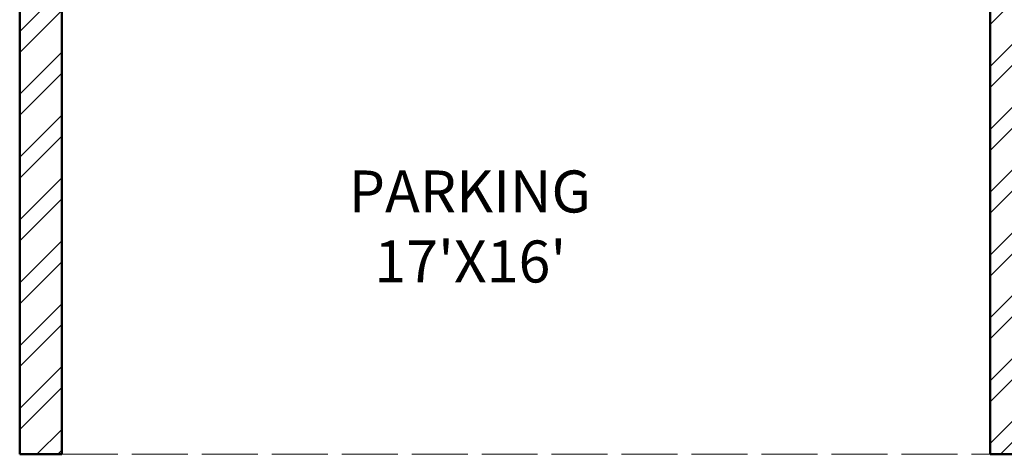
# Model space of a CAD drawing. Units: inches. Extents: x -31485 to -28799, y 18003 to 19130.
# Tile 1 of 15: x -31210 to -30999, y 18180 to 18273. Entities that reach past the tile are written whole.
import ezdxf

# ---------------------------------------------------------------- set-up
doc = ezdxf.new("R2010")
doc.units = ezdxf.units.IN
doc.linetypes.add('ACAD_ISO02W100', pattern=[15, 12, -3])
for name, color, linetype, lineweight in [('A-AREA-IDEN', 7, 'Continuous', 18), ('A-FLOR-OVHD', 30, 'ACAD_ISO02W100', 18), ('A-WALL', 7, 'Continuous', 50), ('A-WALL-PATT', 8, 'Continuous', 13)]:
    doc.layers.add(name, color=color, linetype=linetype, lineweight=lineweight)
doc.styles.get("Standard").update_dxf_attribs({"font": 'arial.ttf'})

msp = doc.modelspace()

# ---------------------------------------------------------------- hatches: boundary and pattern name
at = {"layer": 'A-WALL-PATT'}
h = msp.add_hatch(dxfattribs=at)
h.set_pattern_fill('ANSI32', color=256)
h.set_pattern_definition([(45, (-1687.357050595019, -0.3129728357926069), (-6.735192090801865, 6.735192090801866), []), (45, (-1682.866920595021, -0.3129728357926069), (-6.735192090801865, 6.735192090801866), [])])
h.paths.add_polyline_path([(-31156.52828769349, 18823.80296009311), (-31209.52828769349, 18823.80296009311), (-31209.52828769349, 18761.80296009311), (-31200.52828769349, 18761.80296009311), (-31200.52828769349, 18814.80296009311), (-31156.52828769349, 18814.80296009311)], flags=17)
h.paths.add_polyline_path([(-31022.5282876935, 18823.80296009311), (-31118.52828769349, 18823.80296009311), (-31118.52828769349, 18814.80296009311), (-31074.52828769349, 18814.80296009311), (-31074.52828769349, 18720.78574754094), (-31070.95696393926, 18720.78574754094), (-31068.52828769349, 18720.75952290947), (-31068.52828769349, 18814.80296009311), (-31022.5282876935, 18814.80296009311)], flags=17)
h.paths.add_polyline_path([(-30754.52828769349, 18823.80296009311), (-30850.5282876935, 18823.80296009311), (-30850.5282876935, 18814.80296009311), (-30806.5282876935, 18814.80296009311), (-30806.52828769349, 18723.10029278397), (-30800.5282876935, 18723.10029278397), (-30800.5282876935, 18814.80296009311), (-30754.52828769349, 18814.80296009311)], flags=17)
h.paths.add_polyline_path([(-30661.52828769349, 18823.80296009311), (-30716.52828769349, 18823.80296009311), (-30716.52828769349, 18814.80296009311), (-30670.52828769349, 18814.80296009311), (-30670.52828769349, 18761.80296009311), (-30661.52828769349, 18761.80296009311)], flags=17)
h.paths.add_polyline_path([(-30986.91891278487, 18670.80296009311), (-31068.52828769349, 18670.80296009311), (-31068.52828769349, 18684.75952290947), (-31074.52828769349, 18684.75952290947), (-31074.52828769349, 18670.80296009311), (-31200.52828769349, 18670.80296009311), (-31200.52828769349, 18723.80296009311), (-31209.52828769349, 18723.80296009311), (-31209.52828769349, 18641.80296009311), (-31200.52828769349, 18641.80296009311), (-31200.52828769349, 18664.80296009311), (-31104.52828769349, 18664.80296009311), (-31104.52828769349, 18628.92834044014), (-31098.52828769349, 18628.92834044014), (-31098.52828769348, 18664.8029600931), (-30986.91891278488, 18664.8029600931)], flags=17)
h.paths.add_polyline_path([(-30661.52828769349, 18723.80296009311), (-30670.52828769349, 18723.80296009311), (-30670.52828769349, 18670.80296009311), (-30800.5282876935, 18670.80296009311), (-30800.5282876935, 18687.10029278396), (-30806.52828769349, 18687.10029278396), (-30806.52828769349, 18670.80296009311), (-30885.59628027248, 18670.80296009311), (-30885.59628027248, 18667.80293426455), (-30885.59628027248, 18664.80296009311), (-30760.52828769349, 18664.80296009311), (-30760.52828769349, 18625.80296009311), (-30754.52828769349, 18625.80296009311), (-30754.52828769349, 18664.80296009311), (-30670.52828769349, 18664.80296009311), (-30670.52828769349, 18641.80296009311), (-30661.52828769349, 18641.80296009311)], flags=17)
h.paths.add_polyline_path([(-31200.52828769349, 18574.80296009311), (-31188.56436894977, 18574.80296009311), (-31188.56436894977, 18580.80296009311), (-31200.52828769349, 18580.80296009311), (-31200.52828769349, 18603.80296009311), (-31209.52828769349, 18603.80296009311), (-31209.52828769349, 18557.80296009311), (-31200.52828769349, 18557.80296009311)], flags=17)
h.paths.add_polyline_path([(-31098.52828769349, 18592.92834044014), (-31104.52828769349, 18592.92834044014), (-31104.52828769349, 18580.80296009311), (-31164.56436894977, 18580.80296009311), (-31164.56436894977, 18574.80296009311), (-31104.52828769349, 18574.80296009311), (-31104.52828769349, 18514.80296009311), (-31200.52828769349, 18514.80296009311), (-31200.52828769349, 18531.80296009311), (-31209.52828769349, 18531.80296009311), (-31209.52828769349, 18473.80296009311), (-31200.52828769349, 18473.80296009311), (-31200.52828769349, 18508.80296009311), (-31056.52828769349, 18508.80296009312), (-31056.52828769349, 18501.62307445529), (-31050.52828769349, 18501.62307445529), (-31050.52828769349, 18514.80296009311), (-31098.52828769349, 18514.80296009311)], flags=17)
h.paths.add_polyline_path([(-30661.52828769349, 18531.80296009311), (-30670.52828769349, 18531.80296009311), (-30670.52828769349, 18514.80296009311), (-30754.52828769349, 18514.80296009311), (-30754.52828769349, 18574.80296009311), (-30700.74522746605, 18574.80296009311), (-30700.74522746605, 18577.44024221289), (-30700.74522746605, 18580.8029600931), (-30754.52828769349, 18580.80296009311), (-30754.52828769349, 18589.80296009311), (-30760.52828769349, 18589.80296009311), (-30760.52828769349, 18514.80296009311), (-30820.52828769349, 18514.80296009311), (-30820.52828769348, 18499.26438911774), (-30814.52828769349, 18499.26438911774), (-30814.52828769349, 18508.80296009311), (-30670.52828769349, 18508.80296009311), (-30670.52828769349, 18473.80296009311), (-30661.52828769349, 18473.80296009311)], flags=17)
h.paths.add_polyline_path([(-30661.52828769349, 18435.80296009311), (-30670.52828769349, 18435.80296009311), (-30670.52828769349, 18400.80296009311), (-30814.52828769349, 18400.80296009311), (-30814.52828769349, 18413.15176302367), (-30820.52828769349, 18413.15176302367), (-30820.52828769349, 18400.80296009311), (-30932.52828769349, 18400.80296009311), (-30932.52828769349, 18664.80296009311), (-30921.59628027248, 18664.80296009311), (-30921.59628027248, 18670.80296009311), (-30932.5282876935, 18670.80296009311), (-30932.5282876935, 18814.80296009311), (-30888.5282876935, 18814.80296009311), (-30888.5282876935, 18823.80296009311), (-30984.5282876935, 18823.80296009311), (-30984.5282876935, 18814.80296009311), (-30938.5282876935, 18814.80296009311), (-30938.5282876935, 18670.80296009311), (-30950.91891278487, 18670.80296009311), (-30950.91891278488, 18664.80296009311), (-30938.5282876935, 18664.80296009311), (-30938.52828769349, 18400.80296009311), (-31050.52828769349, 18400.80296009311), (-31050.52828769349, 18411.18080736427), (-31056.52828769348, 18411.18080736427), (-31056.52828769348, 18400.80296009311), (-31200.52828769349, 18400.80296009311), (-31200.52828769349, 18435.80296009311), (-31209.52828769349, 18435.80296009311), (-31209.52828769349, 18179.80296009311), (-31200.52828769349, 18179.80296009311), (-31200.52828769349, 18394.80296009311), (-31001.52828769348, 18394.80296009311), (-31001.52828769348, 18179.80296009311), (-30954.52828769347, 18179.80296009311), (-30954.52828769347, 18188.80296009311), (-30995.52828769348, 18188.80296009311), (-30995.52828769348, 18394.80296009311), (-30875.52828769348, 18394.80296009311), (-30875.52828769348, 18188.80296009311), (-30916.52828769347, 18188.80296009311), (-30916.52828769347, 18179.80296009311), (-30869.52828769348, 18179.80296009311), (-30869.52828769348, 18394.80296009311), (-30670.52828769349, 18394.80296009311), (-30670.52828769349, 18179.80296009311), (-30661.52828769349, 18179.80296009311)])

# ---------------------------------------------------------------- linework, layer by layer
at = {"layer": 'A-FLOR-OVHD'}
msp.add_line((-31200.52828769348, 18179.80296009311), (-31001.52828769348, 18179.80296009311), dxfattribs=at)
at = {"layer": 'A-WALL'}
for p, q in [((-31209.52828769349, 18179.80296009311), (-31209.52828769349, 18823.80296009311)), ((-31200.52828769349, 18179.80296009311), (-31200.52828769349, 18394.80296009311)), ((-31001.52828769348, 18394.80296009311), (-31001.52828769348, 18179.80296009311)), ((-31200.52828769348, 18179.80296009311), (-31209.52828769349, 18179.80296009311)), ((-30869.52828769348, 18179.80296009311), (-31001.52828769348, 18179.80296009311))]:
    msp.add_line(p, q, dxfattribs=at)

# ---------------------------------------------------------------- texts
at = {"layer": 'A-AREA-IDEN', "insert": (-31139.01234277374, 18240.63394989423), "char_height": 9, "attachment_point": 1}
msp.add_mtext_dynamic_manual_height_columns("{PARKING\\P  17'X16'}", width=763.1478888985547, gutter_width=12.5, heights=[0], dxfattribs=at)

doc.saveas('drawing.dxf')
